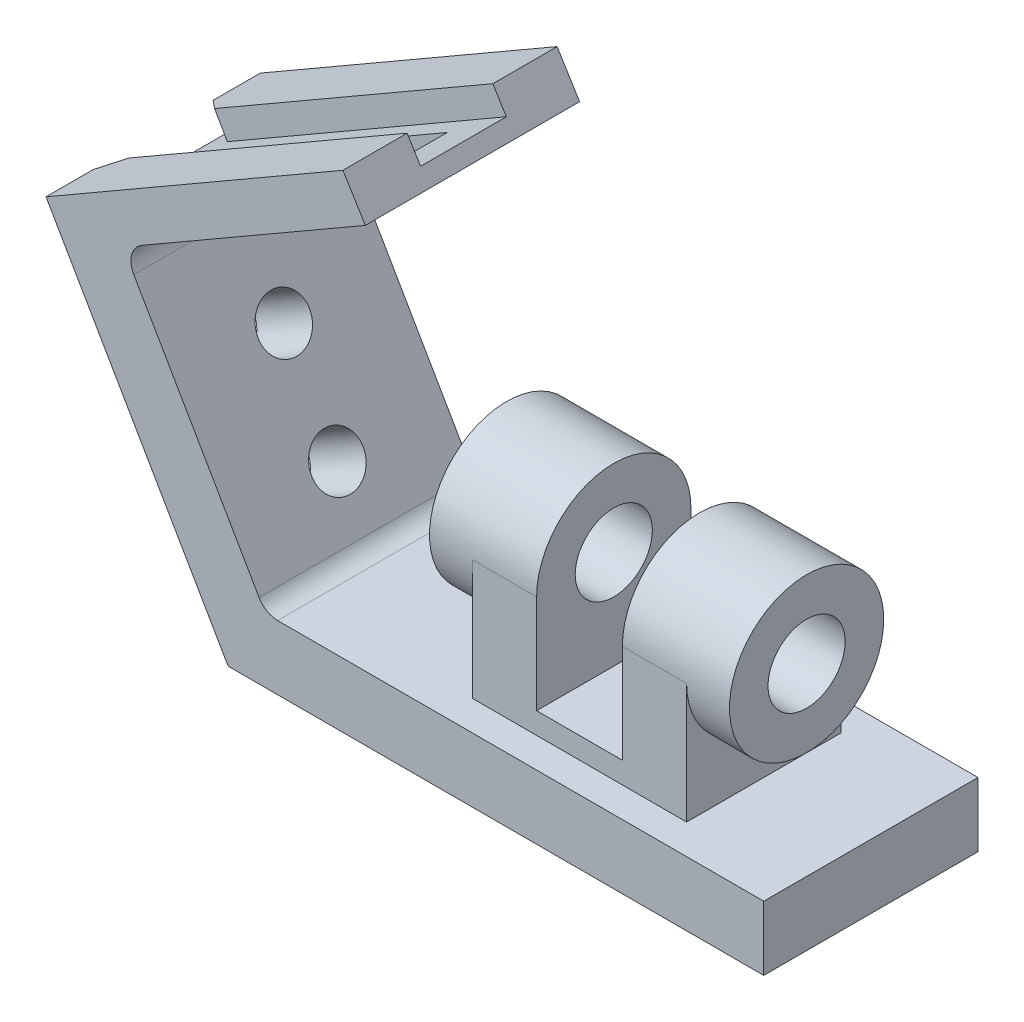
ISO-10303-21;
HEADER;
FILE_DESCRIPTION(('STEP AP214'),'2;1');
FILE_NAME('part.step','',(''),(''),'','','');
FILE_SCHEMA(('AUTOMOTIVE_DESIGN { 1 0 10303 214 1 1 1 1 }'));
ENDSEC;
DATA;
#1=APPLICATION_CONTEXT('core data for automotive mechanical design processes');
#2=APPLICATION_PROTOCOL_DEFINITION('international standard','automotive_design',2000,#1);
#3=PRODUCT_CONTEXT('',#1,'mechanical');
#4=PRODUCT('Part','Part','',(#3));
#5=PRODUCT_RELATED_PRODUCT_CATEGORY('part','',(#4));
#6=PRODUCT_DEFINITION_FORMATION('','',#4);
#7=PRODUCT_DEFINITION_CONTEXT('part definition',#1,'design');
#8=PRODUCT_DEFINITION('design','',#6,#7);
#9=PRODUCT_DEFINITION_SHAPE('','',#8);
#10=(LENGTH_UNIT() NAMED_UNIT(*) SI_UNIT(.MILLI.,.METRE.));
#11=(NAMED_UNIT(*) PLANE_ANGLE_UNIT() SI_UNIT($,.RADIAN.));
#12=(NAMED_UNIT(*) SI_UNIT($,.STERADIAN.) SOLID_ANGLE_UNIT());
#13=UNCERTAINTY_MEASURE_WITH_UNIT(LENGTH_MEASURE(1.E-05),#10,'distance_accuracy_value','');
#14=(GEOMETRIC_REPRESENTATION_CONTEXT(3) GLOBAL_UNCERTAINTY_ASSIGNED_CONTEXT((#13)) GLOBAL_UNIT_ASSIGNED_CONTEXT((#10,
#11,#12)) REPRESENTATION_CONTEXT('',''));
#15=CARTESIAN_POINT('',(0.,0.,0.));
#16=DIRECTION('',(0.,0.,1.));
#17=DIRECTION('',(1.,0.,0.));
#18=AXIS2_PLACEMENT_3D('',#15,#16,#17);
#19=CARTESIAN_POINT('',(40.,43.,0.));
#20=DIRECTION('',(1.,0.,0.));
#21=DIRECTION('',(0.,0.,-1.));
#22=AXIS2_PLACEMENT_3D('',#19,#20,#21);
#23=CYLINDRICAL_SURFACE('',#22,18.);
#24=CARTESIAN_POINT('',(85.,43.,0.));
#25=DIRECTION('',(1.,0.,0.));
#26=DIRECTION('',(0.,1.,0.));
#27=AXIS2_PLACEMENT_3D('',#24,#25,#26);
#28=CIRCLE('',#27,18.);
#29=CARTESIAN_POINT('',(85.,43.,18.));
#30=VERTEX_POINT('',#29);
#31=CARTESIAN_POINT('',(85.,43.,-18.));
#32=VERTEX_POINT('',#31);
#33=EDGE_CURVE('E48',#30,#32,#28,.F.);
#34=ORIENTED_EDGE('',*,*,#33,.F.);
#35=DIRECTION('',(1.,0.,0.));
#36=VECTOR('',#35,1.);
#37=CARTESIAN_POINT('',(50.,43.,18.));
#38=LINE('',#37,#36);
#39=CARTESIAN_POINT('',(100.,43.,18.));
#40=VERTEX_POINT('',#39);
#41=EDGE_CURVE('E285',#30,#40,#38,.T.);
#42=ORIENTED_EDGE('',*,*,#41,.T.);
#43=CARTESIAN_POINT('',(100.,43.,0.));
#44=DIRECTION('',(-1.,0.,0.));
#45=DIRECTION('',(0.,0.,1.));
#46=AXIS2_PLACEMENT_3D('',#43,#44,#45);
#47=CIRCLE('',#46,18.);
#48=CARTESIAN_POINT('',(100.,43.,-18.));
#49=VERTEX_POINT('',#48);
#50=EDGE_CURVE('E434',#49,#40,#47,.T.);
#51=ORIENTED_EDGE('',*,*,#50,.F.);
#52=DIRECTION('',(1.,0.,0.));
#53=VECTOR('',#52,1.);
#54=CARTESIAN_POINT('',(50.,43.,-18.));
#55=LINE('',#54,#53);
#56=EDGE_CURVE('E276',#32,#49,#55,.T.);
#57=ORIENTED_EDGE('',*,*,#56,.F.);
#58=EDGE_LOOP('',(#34,#42,#51,#57));
#59=FACE_BOUND('',#58,.T.);
#60=CARTESIAN_POINT('',(110.,43.,0.));
#61=DIRECTION('',(1.,0.,0.));
#62=DIRECTION('',(0.,0.,-1.));
#63=AXIS2_PLACEMENT_3D('',#60,#61,#62);
#64=CIRCLE('',#63,18.);
#65=CARTESIAN_POINT('',(110.,43.,-18.));
#66=VERTEX_POINT('',#65);
#67=EDGE_CURVE('E255',#66,#66,#64,.T.);
#68=ORIENTED_EDGE('',*,*,#67,.F.);
#69=EDGE_LOOP('',(#68));
#70=FACE_BOUND('',#69,.T.);
#71=ADVANCED_FACE('F39',(#59,#70),#23,.T.);
#72=CARTESIAN_POINT('',(-42.5000000000004,73.6121593216771,25.));
#73=DIRECTION('',(0.500000000000004,-0.866025403784436,0.));
#74=DIRECTION('',(0.866025403784436,0.500000000000004,0.));
#75=AXIS2_PLACEMENT_3D('',#72,#73,#74);
#76=PLANE('',#75);
#77=DIRECTION('',(0.,0.,-1.));
#78=VECTOR('',#77,1.);
#79=CARTESIAN_POINT('',(-42.5000000000004,73.6121593216771,25.));
#80=LINE('',#79,#78);
#81=CARTESIAN_POINT('',(-42.5000000000004,73.6121593216771,-14.));
#82=VERTEX_POINT('',#81);
#83=CARTESIAN_POINT('',(-42.5000000000004,73.6121593216771,-25.));
#84=VERTEX_POINT('',#83);
#85=EDGE_CURVE('E410',#82,#84,#80,.T.);
#86=ORIENTED_EDGE('',*,*,#85,.F.);
#87=DIRECTION('',(-0.676252226000572,-0.39043440472152,-0.624695047554424));
#88=VECTOR('',#87,1.);
#89=CARTESIAN_POINT('',(-42.5000000000004,73.6121593216771,-14.));
#90=LINE('',#89,#88);
#91=CARTESIAN_POINT('',(-38.1698729810782,76.1121593216771,-10.));
#92=VERTEX_POINT('',#91);
#93=EDGE_CURVE('E316',#92,#82,#90,.T.);
#94=ORIENTED_EDGE('',*,*,#93,.F.);
#95=DIRECTION('',(0.866025403784436,0.500000000000004,0.));
#96=VECTOR('',#95,1.);
#97=CARTESIAN_POINT('',(-38.1698729810782,76.1121593216771,-10.));
#98=LINE('',#97,#96);
#99=CARTESIAN_POINT('',(26.7820323027545,113.612159321677,-10.));
#100=VERTEX_POINT('',#99);
#101=EDGE_CURVE('E342',#92,#100,#98,.T.);
#102=ORIENTED_EDGE('',*,*,#101,.T.);
#103=DIRECTION('',(0.,0.,-1.));
#104=VECTOR('',#103,1.);
#105=CARTESIAN_POINT('',(26.7820323027545,113.612159321677,25.));
#106=LINE('',#105,#104);
#107=CARTESIAN_POINT('',(26.7820323027545,113.612159321677,-25.));
#108=VERTEX_POINT('',#107);
#109=EDGE_CURVE('E414',#100,#108,#106,.T.);
#110=ORIENTED_EDGE('',*,*,#109,.T.);
#111=DIRECTION('',(-0.866025403784436,-0.500000000000004,0.));
#112=VECTOR('',#111,1.);
#113=CARTESIAN_POINT('',(-42.5000000000004,73.6121593216771,-25.));
#114=LINE('',#113,#112);
#115=EDGE_CURVE('E396',#108,#84,#114,.T.);
#116=ORIENTED_EDGE('',*,*,#115,.T.);
#117=EDGE_LOOP('',(#86,#94,#102,#110,#116));
#118=FACE_BOUND('',#117,.T.);
#119=ADVANCED_FACE('F478',(#118),#76,.F.);
#120=CARTESIAN_POINT('',(32.0205297038397,105.094052432302,25.));
#121=DIRECTION('',(-0.851810688937537,-0.523849740108516,0.));
#122=DIRECTION('',(0.523849740108516,-0.851810688937537,0.));
#123=AXIS2_PLACEMENT_3D('',#120,#121,#122);
#124=PLANE('',#123);
#125=DIRECTION('',(-0.523849740108516,0.851810688937537,0.));
#126=VECTOR('',#125,1.);
#127=CARTESIAN_POINT('',(32.0205297038397,105.094052432302,-9.99999999999999));
#128=LINE('',#127,#126);
#129=CARTESIAN_POINT('',(29.926342667875,108.49932452712,-10.));
#130=VERTEX_POINT('',#129);
#131=EDGE_CURVE('E355',#130,#100,#128,.T.);
#132=ORIENTED_EDGE('',*,*,#131,.F.);
#133=DIRECTION('',(0.,0.,-1.));
#134=VECTOR('',#133,1.);
#135=CARTESIAN_POINT('',(29.926342667875,108.49932452712,25.));
#136=LINE('',#135,#134);
#137=CARTESIAN_POINT('',(29.926342667875,108.49932452712,10.));
#138=VERTEX_POINT('',#137);
#139=EDGE_CURVE('E433',#138,#130,#136,.T.);
#140=ORIENTED_EDGE('',*,*,#139,.F.);
#141=DIRECTION('',(-0.523849740108516,0.851810688937537,0.));
#142=VECTOR('',#141,1.);
#143=CARTESIAN_POINT('',(32.0205297038397,105.094052432302,10.));
#144=LINE('',#143,#142);
#145=CARTESIAN_POINT('',(26.7820323027545,113.612159321677,10.));
#146=VERTEX_POINT('',#145);
#147=EDGE_CURVE('E347',#138,#146,#144,.T.);
#148=ORIENTED_EDGE('',*,*,#147,.T.);
#149=CARTESIAN_POINT('',(26.7820323027545,113.612159321677,25.));
#150=VERTEX_POINT('',#149);
#151=EDGE_CURVE('E411',#150,#146,#106,.T.);
#152=ORIENTED_EDGE('',*,*,#151,.F.);
#153=DIRECTION('',(-0.523849740108516,0.851810688937537,0.));
#154=VECTOR('',#153,1.);
#155=CARTESIAN_POINT('',(32.0205297038397,105.094052432302,25.));
#156=LINE('',#155,#154);
#157=CARTESIAN_POINT('',(32.0205297038397,105.094052432302,25.));
#158=VERTEX_POINT('',#157);
#159=EDGE_CURVE('E375',#158,#150,#156,.T.);
#160=ORIENTED_EDGE('',*,*,#159,.F.);
#161=DIRECTION('',(0.,0.,-1.));
#162=VECTOR('',#161,1.);
#163=CARTESIAN_POINT('',(32.0205297038397,105.094052432302,25.));
#164=LINE('',#163,#162);
#165=CARTESIAN_POINT('',(32.0205297038397,105.094052432302,-25.));
#166=VERTEX_POINT('',#165);
#167=EDGE_CURVE('E412',#158,#166,#164,.T.);
#168=ORIENTED_EDGE('',*,*,#167,.T.);
#169=DIRECTION('',(-0.523849740108516,0.851810688937537,0.));
#170=VECTOR('',#169,1.);
#171=CARTESIAN_POINT('',(32.0205297038397,105.094052432302,-25.));
#172=LINE('',#171,#170);
#173=EDGE_CURVE('E395',#166,#108,#172,.T.);
#174=ORIENTED_EDGE('',*,*,#173,.T.);
#175=ORIENTED_EDGE('',*,*,#109,.F.);
#176=EDGE_LOOP('',(#132,#140,#148,#152,#160,#168,#174,#175));
#177=FACE_BOUND('',#176,.T.);
#178=ADVANCED_FACE('F485',(#177),#124,.F.);
#179=DIRECTION('',(0.866025403784436,0.500000000000004,0.));
#180=VECTOR('',#179,1.);
#181=CARTESIAN_POINT('',(-38.1698729810782,76.1121593216771,10.));
#182=LINE('',#181,#180);
#183=CARTESIAN_POINT('',(-38.1698729810782,76.1121593216771,10.));
#184=VERTEX_POINT('',#183);
#185=EDGE_CURVE('E333',#184,#146,#182,.T.);
#186=ORIENTED_EDGE('',*,*,#185,.F.);
#187=DIRECTION('',(0.676252226000572,0.390434404721518,-0.624695047554425));
#188=VECTOR('',#187,1.);
#189=CARTESIAN_POINT('',(-38.1698729810782,76.1121593216771,10.));
#190=LINE('',#189,#188);
#191=CARTESIAN_POINT('',(-42.5000000000004,73.6121593216771,14.));
#192=VERTEX_POINT('',#191);
#193=EDGE_CURVE('E321',#192,#184,#190,.T.);
#194=ORIENTED_EDGE('',*,*,#193,.F.);
#195=CARTESIAN_POINT('',(-42.5000000000004,73.6121593216771,25.));
#196=VERTEX_POINT('',#195);
#197=EDGE_CURVE('E409',#196,#192,#80,.T.);
#198=ORIENTED_EDGE('',*,*,#197,.F.);
#199=DIRECTION('',(-0.866025403784436,-0.500000000000004,0.));
#200=VECTOR('',#199,1.);
#201=CARTESIAN_POINT('',(-42.5000000000004,73.6121593216771,25.));
#202=LINE('',#201,#200);
#203=EDGE_CURVE('E372',#150,#196,#202,.T.);
#204=ORIENTED_EDGE('',*,*,#203,.F.);
#205=ORIENTED_EDGE('',*,*,#151,.T.);
#206=EDGE_LOOP('',(#186,#194,#198,#204,#205));
#207=FACE_BOUND('',#206,.T.);
#208=ADVANCED_FACE('F486',(#207),#76,.F.);
#209=CARTESIAN_POINT('',(125.,0.,25.));
#210=DIRECTION('',(-1.,0.,0.));
#211=DIRECTION('',(0.,0.,1.));
#212=AXIS2_PLACEMENT_3D('',#209,#210,#211);
#213=PLANE('',#212);
#214=DIRECTION('',(0.,1.,0.));
#215=VECTOR('',#214,1.);
#216=CARTESIAN_POINT('',(125.,0.,-25.));
#217=LINE('',#216,#215);
#218=CARTESIAN_POINT('',(125.,0.,-25.));
#219=VERTEX_POINT('',#218);
#220=CARTESIAN_POINT('',(125.,15.,-25.));
#221=VERTEX_POINT('',#220);
#222=EDGE_CURVE('E357',#219,#221,#217,.T.);
#223=ORIENTED_EDGE('',*,*,#222,.T.);
#224=DIRECTION('',(0.,0.,-1.));
#225=VECTOR('',#224,1.);
#226=CARTESIAN_POINT('',(125.,15.,25.));
#227=LINE('',#226,#225);
#228=CARTESIAN_POINT('',(125.,15.,25.));
#229=VERTEX_POINT('',#228);
#230=EDGE_CURVE('E427',#229,#221,#227,.T.);
#231=ORIENTED_EDGE('',*,*,#230,.F.);
#232=DIRECTION('',(0.,1.,0.));
#233=VECTOR('',#232,1.);
#234=CARTESIAN_POINT('',(125.,0.,25.));
#235=LINE('',#234,#233);
#236=CARTESIAN_POINT('',(125.,0.,25.));
#237=VERTEX_POINT('',#236);
#238=EDGE_CURVE('E356',#237,#229,#235,.T.);
#239=ORIENTED_EDGE('',*,*,#238,.F.);
#240=DIRECTION('',(0.,0.,-1.));
#241=VECTOR('',#240,1.);
#242=CARTESIAN_POINT('',(125.,0.,25.));
#243=LINE('',#242,#241);
#244=EDGE_CURVE('E379',#237,#219,#243,.T.);
#245=ORIENTED_EDGE('',*,*,#244,.T.);
#246=EDGE_LOOP('',(#223,#231,#239,#245));
#247=FACE_BOUND('',#246,.T.);
#248=ADVANCED_FACE('F41',(#247),#213,.F.);
#249=CARTESIAN_POINT('',(125.,15.,25.));
#250=DIRECTION('',(0.,-1.,0.));
#251=DIRECTION('',(1.,0.,0.));
#252=AXIS2_PLACEMENT_3D('',#249,#250,#251);
#253=PLANE('',#252);
#254=DIRECTION('',(1.,0.,0.));
#255=VECTOR('',#254,1.);
#256=CARTESIAN_POINT('',(50.,15.,18.));
#257=LINE('',#256,#255);
#258=CARTESIAN_POINT('',(50.,15.,18.));
#259=VERTEX_POINT('',#258);
#260=CARTESIAN_POINT('',(100.,15.,18.));
#261=VERTEX_POINT('',#260);
#262=EDGE_CURVE('E64',#259,#261,#257,.T.);
#263=ORIENTED_EDGE('',*,*,#262,.F.);
#264=DIRECTION('',(0.,0.,1.));
#265=VECTOR('',#264,1.);
#266=CARTESIAN_POINT('',(50.,15.,-18.));
#267=LINE('',#266,#265);
#268=CARTESIAN_POINT('',(50.,15.,-18.));
#269=VERTEX_POINT('',#268);
#270=EDGE_CURVE('E264',#269,#259,#267,.T.);
#271=ORIENTED_EDGE('',*,*,#270,.F.);
#272=DIRECTION('',(1.,0.,0.));
#273=VECTOR('',#272,1.);
#274=CARTESIAN_POINT('',(50.,15.,-18.));
#275=LINE('',#274,#273);
#276=CARTESIAN_POINT('',(100.,15.,-18.));
#277=VERTEX_POINT('',#276);
#278=EDGE_CURVE('E272',#269,#277,#275,.T.);
#279=ORIENTED_EDGE('',*,*,#278,.T.);
#280=DIRECTION('',(0.,0.,1.));
#281=VECTOR('',#280,1.);
#282=CARTESIAN_POINT('',(100.,15.,-18.));
#283=LINE('',#282,#281);
#284=EDGE_CURVE('E258',#277,#261,#283,.T.);
#285=ORIENTED_EDGE('',*,*,#284,.T.);
#286=EDGE_LOOP('',(#263,#271,#279,#285));
#287=FACE_BOUND('',#286,.T.);
#288=DIRECTION('',(-1.,0.,0.));
#289=VECTOR('',#288,1.);
#290=CARTESIAN_POINT('',(125.,15.,-25.));
#291=LINE('',#290,#289);
#292=CARTESIAN_POINT('',(11.5470053837925,15.,-25.));
#293=VERTEX_POINT('',#292);
#294=EDGE_CURVE('E384',#221,#293,#291,.T.);
#295=ORIENTED_EDGE('',*,*,#294,.T.);
#296=DIRECTION('',(0.,0.,-1.));
#297=VECTOR('',#296,1.);
#298=CARTESIAN_POINT('',(11.5470053837925,15.,25.));
#299=LINE('',#298,#297);
#300=CARTESIAN_POINT('',(11.5470053837925,15.,25.));
#301=VERTEX_POINT('',#300);
#302=EDGE_CURVE('E430',#301,#293,#299,.T.);
#303=ORIENTED_EDGE('',*,*,#302,.F.);
#304=DIRECTION('',(-1.,0.,0.));
#305=VECTOR('',#304,1.);
#306=CARTESIAN_POINT('',(125.,15.,25.));
#307=LINE('',#306,#305);
#308=EDGE_CURVE('E363',#229,#301,#307,.T.);
#309=ORIENTED_EDGE('',*,*,#308,.F.);
#310=ORIENTED_EDGE('',*,*,#230,.T.);
#311=EDGE_LOOP('',(#295,#303,#309,#310));
#312=FACE_BOUND('',#311,.T.);
#313=ADVANCED_FACE('F570',(#287,#312),#253,.F.);
#314=CARTESIAN_POINT('',(11.5470053837924,20.,25.));
#315=DIRECTION('',(0.,0.,-1.));
#316=DIRECTION('',(-1.,0.,0.));
#317=AXIS2_PLACEMENT_3D('',#314,#315,#316);
#318=CYLINDRICAL_SURFACE('',#317,5.);
#319=CARTESIAN_POINT('',(11.5470053837924,20.,-25.));
#320=DIRECTION('',(0.,0.,-1.));
#321=DIRECTION('',(-1.,0.,0.));
#322=AXIS2_PLACEMENT_3D('',#319,#320,#321);
#323=CIRCLE('',#322,5.);
#324=CARTESIAN_POINT('',(7.21687836487027,17.5,-25.));
#325=VERTEX_POINT('',#324);
#326=EDGE_CURVE('E383',#293,#325,#323,.T.);
#327=ORIENTED_EDGE('',*,*,#326,.T.);
#328=DIRECTION('',(0.,0.,-1.));
#329=VECTOR('',#328,1.);
#330=CARTESIAN_POINT('',(7.21687836487027,17.5,25.));
#331=LINE('',#330,#329);
#332=CARTESIAN_POINT('',(7.21687836487027,17.5,25.));
#333=VERTEX_POINT('',#332);
#334=EDGE_CURVE('E425',#333,#325,#331,.T.);
#335=ORIENTED_EDGE('',*,*,#334,.F.);
#336=CARTESIAN_POINT('',(11.5470053837924,20.,25.));
#337=DIRECTION('',(0.,0.,-1.));
#338=DIRECTION('',(-1.,0.,0.));
#339=AXIS2_PLACEMENT_3D('',#336,#337,#338);
#340=CIRCLE('',#339,5.);
#341=EDGE_CURVE('E364',#301,#333,#340,.T.);
#342=ORIENTED_EDGE('',*,*,#341,.F.);
#343=ORIENTED_EDGE('',*,*,#302,.T.);
#344=EDGE_LOOP('',(#327,#335,#342,#343));
#345=FACE_BOUND('',#344,.T.);
#346=ADVANCED_FACE('F562',(#345),#318,.F.);
#347=CARTESIAN_POINT('',(7.21687836487027,17.5,25.));
#348=DIRECTION('',(-0.866025403784436,-0.500000000000004,0.));
#349=DIRECTION('',(0.500000000000004,-0.866025403784436,0.));
#350=AXIS2_PLACEMENT_3D('',#347,#348,#349);
#351=PLANE('',#350);
#352=CARTESIAN_POINT('',(0.49038105676642,29.150635094611,0.));
#353=DIRECTION('',(-0.866025403784436,-0.500000000000004,0.));
#354=DIRECTION('',(0.500000000000004,-0.866025403784436,0.));
#355=AXIS2_PLACEMENT_3D('',#352,#353,#354);
#356=CIRCLE('',#355,6.);
#357=CARTESIAN_POINT('',(3.49038105676645,23.9544826719044,0.));
#358=VERTEX_POINT('',#357);
#359=EDGE_CURVE('E835',#358,#358,#356,.T.);
#360=ORIENTED_EDGE('',*,*,#359,.T.);
#361=EDGE_LOOP('',(#360));
#362=FACE_BOUND('',#361,.T.);
#363=CARTESIAN_POINT('',(-12.0096189432337,50.8012701892219,0.));
#364=DIRECTION('',(-0.866025403784436,-0.500000000000004,0.));
#365=DIRECTION('',(0.500000000000004,-0.866025403784436,0.));
#366=AXIS2_PLACEMENT_3D('',#363,#364,#365);
#367=CIRCLE('',#366,6.);
#368=CARTESIAN_POINT('',(-9.00961894323366,45.6051177665153,0.));
#369=VERTEX_POINT('',#368);
#370=EDGE_CURVE('E833',#369,#369,#367,.T.);
#371=ORIENTED_EDGE('',*,*,#370,.T.);
#372=EDGE_LOOP('',(#371));
#373=FACE_BOUND('',#372,.T.);
#374=DIRECTION('',(-0.500000000000004,0.866025403784436,0.));
#375=VECTOR('',#374,1.);
#376=CARTESIAN_POINT('',(7.21687836487027,17.5,-25.));
#377=LINE('',#376,#375);
#378=CARTESIAN_POINT('',(-22.0115461137875,68.1251162222244,-25.));
#379=VERTEX_POINT('',#378);
#380=EDGE_CURVE('E390',#325,#379,#377,.T.);
#381=ORIENTED_EDGE('',*,*,#380,.T.);
#382=DIRECTION('',(0.,0.,-1.));
#383=VECTOR('',#382,1.);
#384=CARTESIAN_POINT('',(-22.0115461137875,68.1251162222244,25.));
#385=LINE('',#384,#383);
#386=CARTESIAN_POINT('',(-22.0115461137875,68.1251162222244,25.));
#387=VERTEX_POINT('',#386);
#388=EDGE_CURVE('E423',#387,#379,#385,.T.);
#389=ORIENTED_EDGE('',*,*,#388,.F.);
#390=DIRECTION('',(-0.500000000000004,0.866025403784436,0.));
#391=VECTOR('',#390,1.);
#392=CARTESIAN_POINT('',(7.21687836487027,17.5,25.));
#393=LINE('',#392,#391);
#394=EDGE_CURVE('E366',#333,#387,#393,.T.);
#395=ORIENTED_EDGE('',*,*,#394,.F.);
#396=ORIENTED_EDGE('',*,*,#334,.T.);
#397=EDGE_LOOP('',(#381,#389,#395,#396));
#398=FACE_BOUND('',#397,.T.);
#399=ADVANCED_FACE('F557',(#362,#373,#398),#351,.F.);
#400=CARTESIAN_POINT('',(-17.6814190948651,70.6251162222242,25.));
#401=DIRECTION('',(0.,0.,-1.));
#402=DIRECTION('',(-1.,0.,0.));
#403=AXIS2_PLACEMENT_3D('',#400,#401,#402);
#404=CYLINDRICAL_SURFACE('',#403,5.0000000000001);
#405=CARTESIAN_POINT('',(-17.6814190948651,70.6251162222242,-25.));
#406=DIRECTION('',(0.,0.,-1.));
#407=DIRECTION('',(-1.,0.,0.));
#408=AXIS2_PLACEMENT_3D('',#405,#406,#407);
#409=CIRCLE('',#408,5.0000000000001);
#410=CARTESIAN_POINT('',(-20.1814190948653,74.9552432411466,-25.));
#411=VERTEX_POINT('',#410);
#412=EDGE_CURVE('E386',#379,#411,#409,.T.);
#413=ORIENTED_EDGE('',*,*,#412,.T.);
#414=DIRECTION('',(0.,0.,-1.));
#415=VECTOR('',#414,1.);
#416=CARTESIAN_POINT('',(-20.1814190948653,74.9552432411466,25.));
#417=LINE('',#416,#415);
#418=CARTESIAN_POINT('',(-20.1814190948653,74.9552432411466,25.));
#419=VERTEX_POINT('',#418);
#420=EDGE_CURVE('E419',#419,#411,#417,.T.);
#421=ORIENTED_EDGE('',*,*,#420,.F.);
#422=CARTESIAN_POINT('',(-17.6814190948651,70.6251162222242,25.));
#423=DIRECTION('',(0.,0.,-1.));
#424=DIRECTION('',(-1.,0.,0.));
#425=AXIS2_PLACEMENT_3D('',#422,#423,#424);
#426=CIRCLE('',#425,5.0000000000001);
#427=EDGE_CURVE('E368',#387,#419,#426,.T.);
#428=ORIENTED_EDGE('',*,*,#427,.F.);
#429=ORIENTED_EDGE('',*,*,#388,.T.);
#430=EDGE_LOOP('',(#413,#421,#428,#429));
#431=FACE_BOUND('',#430,.T.);
#432=ADVANCED_FACE('F558',(#431),#404,.F.);
#433=CARTESIAN_POINT('',(-20.1814190948653,74.9552432411466,25.));
#434=DIRECTION('',(-0.500000000000001,0.866025403784438,0.));
#435=DIRECTION('',(-0.866025403784438,-0.500000000000001,0.));
#436=AXIS2_PLACEMENT_3D('',#433,#434,#435);
#437=PLANE('',#436);
#438=DIRECTION('',(0.866025403784438,0.500000000000001,0.));
#439=VECTOR('',#438,1.);
#440=CARTESIAN_POINT('',(-20.1814190948653,74.9552432411466,5.));
#441=LINE('',#440,#439);
#442=CARTESIAN_POINT('',(-11.5211650570209,79.9552432411466,5.));
#443=VERTEX_POINT('',#442);
#444=CARTESIAN_POINT('',(23.1198510943566,99.9552432411466,5.00000000000001));
#445=VERTEX_POINT('',#444);
#446=EDGE_CURVE('E312',#443,#445,#441,.T.);
#447=ORIENTED_EDGE('',*,*,#446,.T.);
#448=DIRECTION('',(0.,0.,-1.));
#449=VECTOR('',#448,1.);
#450=CARTESIAN_POINT('',(23.1198510943566,99.9552432411466,25.));
#451=LINE('',#450,#449);
#452=CARTESIAN_POINT('',(23.1198510943566,99.9552432411466,-4.99999999999999));
#453=VERTEX_POINT('',#452);
#454=EDGE_CURVE('E317',#445,#453,#451,.T.);
#455=ORIENTED_EDGE('',*,*,#454,.T.);
#456=DIRECTION('',(-0.866025403784438,-0.500000000000001,0.));
#457=VECTOR('',#456,1.);
#458=CARTESIAN_POINT('',(-20.1814190948653,74.9552432411466,-5.));
#459=LINE('',#458,#457);
#460=CARTESIAN_POINT('',(-11.5211650570209,79.9552432411466,-5.));
#461=VERTEX_POINT('',#460);
#462=EDGE_CURVE('E301',#453,#461,#459,.T.);
#463=ORIENTED_EDGE('',*,*,#462,.T.);
#464=DIRECTION('',(0.,0.,1.));
#465=VECTOR('',#464,1.);
#466=CARTESIAN_POINT('',(-11.5211650570209,79.9552432411466,25.));
#467=LINE('',#466,#465);
#468=EDGE_CURVE('E309',#461,#443,#467,.T.);
#469=ORIENTED_EDGE('',*,*,#468,.T.);
#470=EDGE_LOOP('',(#447,#455,#463,#469));
#471=FACE_BOUND('',#470,.T.);
#472=DIRECTION('',(0.866025403784438,0.500000000000001,0.));
#473=VECTOR('',#472,1.);
#474=CARTESIAN_POINT('',(-20.1814190948653,74.9552432411466,-25.));
#475=LINE('',#474,#473);
#476=EDGE_CURVE('E394',#411,#166,#475,.T.);
#477=ORIENTED_EDGE('',*,*,#476,.T.);
#478=ORIENTED_EDGE('',*,*,#167,.F.);
#479=DIRECTION('',(0.866025403784438,0.500000000000001,0.));
#480=VECTOR('',#479,1.);
#481=CARTESIAN_POINT('',(-20.1814190948653,74.9552432411466,25.));
#482=LINE('',#481,#480);
#483=EDGE_CURVE('E369',#419,#158,#482,.T.);
#484=ORIENTED_EDGE('',*,*,#483,.F.);
#485=ORIENTED_EDGE('',*,*,#420,.T.);
#486=EDGE_LOOP('',(#477,#478,#484,#485));
#487=FACE_BOUND('',#486,.T.);
#488=ADVANCED_FACE('F546',(#471,#487),#437,.F.);
#489=CARTESIAN_POINT('',(0.,0.,25.));
#490=DIRECTION('',(0.866025403784436,0.500000000000004,0.));
#491=DIRECTION('',(-0.500000000000004,0.866025403784436,0.));
#492=AXIS2_PLACEMENT_3D('',#489,#490,#491);
#493=PLANE('',#492);
#494=CARTESIAN_POINT('',(-12.5000000000001,21.6506350946109,0.));
#495=DIRECTION('',(-0.866025403784436,-0.500000000000004,0.));
#496=DIRECTION('',(0.500000000000004,-0.866025403784436,0.));
#497=AXIS2_PLACEMENT_3D('',#494,#495,#496);
#498=CIRCLE('',#497,6.);
#499=CARTESIAN_POINT('',(-9.50000000000009,16.4544826719043,0.));
#500=VERTEX_POINT('',#499);
#501=EDGE_CURVE('E827',#500,#500,#498,.T.);
#502=ORIENTED_EDGE('',*,*,#501,.F.);
#503=EDGE_LOOP('',(#502));
#504=FACE_BOUND('',#503,.T.);
#505=CARTESIAN_POINT('',(-25.0000000000002,43.3012701892218,0.));
#506=DIRECTION('',(-0.866025403784436,-0.500000000000004,0.));
#507=DIRECTION('',(0.500000000000004,-0.866025403784436,0.));
#508=AXIS2_PLACEMENT_3D('',#505,#506,#507);
#509=CIRCLE('',#508,6.);
#510=CARTESIAN_POINT('',(-22.0000000000002,38.1051177665152,0.));
#511=VERTEX_POINT('',#510);
#512=EDGE_CURVE('E836',#511,#511,#509,.T.);
#513=ORIENTED_EDGE('',*,*,#512,.F.);
#514=EDGE_LOOP('',(#513));
#515=FACE_BOUND('',#514,.T.);
#516=DIRECTION('',(0.,0.,1.));
#517=VECTOR('',#516,1.);
#518=CARTESIAN_POINT('',(-39.5000000000003,68.4160068989705,-14.));
#519=LINE('',#518,#517);
#520=CARTESIAN_POINT('',(-39.5000000000003,68.4160068989705,-14.));
#521=VERTEX_POINT('',#520);
#522=CARTESIAN_POINT('',(-39.5000000000003,68.4160068989705,14.));
#523=VERTEX_POINT('',#522);
#524=EDGE_CURVE('E324',#521,#523,#519,.T.);
#525=ORIENTED_EDGE('',*,*,#524,.F.);
#526=DIRECTION('',(-0.500000000000004,0.866025403784436,0.));
#527=VECTOR('',#526,1.);
#528=CARTESIAN_POINT('',(-39.5000000000003,68.4160068989705,-14.));
#529=LINE('',#528,#527);
#530=EDGE_CURVE('E328',#521,#82,#529,.T.);
#531=ORIENTED_EDGE('',*,*,#530,.T.);
#532=ORIENTED_EDGE('',*,*,#85,.T.);
#533=DIRECTION('',(0.500000000000004,-0.866025403784436,0.));
#534=VECTOR('',#533,1.);
#535=CARTESIAN_POINT('',(0.,0.,-25.));
#536=LINE('',#535,#534);
#537=CARTESIAN_POINT('',(0.,0.,-25.));
#538=VERTEX_POINT('',#537);
#539=EDGE_CURVE('E398',#84,#538,#536,.T.);
#540=ORIENTED_EDGE('',*,*,#539,.T.);
#541=DIRECTION('',(0.,0.,-1.));
#542=VECTOR('',#541,1.);
#543=CARTESIAN_POINT('',(0.,0.,25.));
#544=LINE('',#543,#542);
#545=CARTESIAN_POINT('',(0.,0.,25.));
#546=VERTEX_POINT('',#545);
#547=EDGE_CURVE('E404',#546,#538,#544,.T.);
#548=ORIENTED_EDGE('',*,*,#547,.F.);
#549=DIRECTION('',(0.500000000000004,-0.866025403784436,0.));
#550=VECTOR('',#549,1.);
#551=CARTESIAN_POINT('',(0.,0.,25.));
#552=LINE('',#551,#550);
#553=EDGE_CURVE('E376',#196,#546,#552,.T.);
#554=ORIENTED_EDGE('',*,*,#553,.F.);
#555=ORIENTED_EDGE('',*,*,#197,.T.);
#556=DIRECTION('',(-0.500000000000004,0.866025403784436,0.));
#557=VECTOR('',#556,1.);
#558=CARTESIAN_POINT('',(-39.5000000000003,68.4160068989705,14.));
#559=LINE('',#558,#557);
#560=EDGE_CURVE('E332',#523,#192,#559,.T.);
#561=ORIENTED_EDGE('',*,*,#560,.F.);
#562=EDGE_LOOP('',(#525,#531,#532,#540,#548,#554,#555,#561));
#563=FACE_BOUND('',#562,.T.);
#564=ADVANCED_FACE('F545',(#504,#515,#563),#493,.F.);
#565=CARTESIAN_POINT('',(125.,0.,25.));
#566=DIRECTION('',(0.,1.,0.));
#567=DIRECTION('',(0.,0.,1.));
#568=AXIS2_PLACEMENT_3D('',#565,#566,#567);
#569=PLANE('',#568);
#570=DIRECTION('',(1.,0.,0.));
#571=VECTOR('',#570,1.);
#572=CARTESIAN_POINT('',(125.,0.,-25.));
#573=LINE('',#572,#571);
#574=EDGE_CURVE('E365',#538,#219,#573,.T.);
#575=ORIENTED_EDGE('',*,*,#574,.T.);
#576=ORIENTED_EDGE('',*,*,#244,.F.);
#577=DIRECTION('',(1.,0.,0.));
#578=VECTOR('',#577,1.);
#579=CARTESIAN_POINT('',(125.,0.,25.));
#580=LINE('',#579,#578);
#581=EDGE_CURVE('E377',#546,#237,#580,.T.);
#582=ORIENTED_EDGE('',*,*,#581,.F.);
#583=ORIENTED_EDGE('',*,*,#547,.T.);
#584=EDGE_LOOP('',(#575,#576,#582,#583));
#585=FACE_BOUND('',#584,.T.);
#586=ADVANCED_FACE('F537',(#585),#569,.F.);
#587=CARTESIAN_POINT('',(11.5470053837924,20.,25.));
#588=DIRECTION('',(0.,0.,-1.));
#589=DIRECTION('',(-1.,0.,0.));
#590=AXIS2_PLACEMENT_3D('',#587,#588,#589);
#591=PLANE('',#590);
#592=ORIENTED_EDGE('',*,*,#238,.T.);
#593=ORIENTED_EDGE('',*,*,#308,.T.);
#594=ORIENTED_EDGE('',*,*,#341,.T.);
#595=ORIENTED_EDGE('',*,*,#394,.T.);
#596=ORIENTED_EDGE('',*,*,#427,.T.);
#597=ORIENTED_EDGE('',*,*,#483,.T.);
#598=ORIENTED_EDGE('',*,*,#159,.T.);
#599=ORIENTED_EDGE('',*,*,#203,.T.);
#600=ORIENTED_EDGE('',*,*,#553,.T.);
#601=ORIENTED_EDGE('',*,*,#581,.T.);
#602=EDGE_LOOP('',(#592,#593,#594,#595,#596,#597,#598,#599,#600,#601));
#603=FACE_BOUND('',#602,.T.);
#604=ADVANCED_FACE('F531',(#603),#591,.F.);
#605=CARTESIAN_POINT('',(11.5470053837924,20.,-25.));
#606=DIRECTION('',(0.,0.,-1.));
#607=DIRECTION('',(-1.,0.,0.));
#608=AXIS2_PLACEMENT_3D('',#605,#606,#607);
#609=PLANE('',#608);
#610=ORIENTED_EDGE('',*,*,#222,.F.);
#611=ORIENTED_EDGE('',*,*,#574,.F.);
#612=ORIENTED_EDGE('',*,*,#539,.F.);
#613=ORIENTED_EDGE('',*,*,#115,.F.);
#614=ORIENTED_EDGE('',*,*,#173,.F.);
#615=ORIENTED_EDGE('',*,*,#476,.F.);
#616=ORIENTED_EDGE('',*,*,#412,.F.);
#617=ORIENTED_EDGE('',*,*,#380,.F.);
#618=ORIENTED_EDGE('',*,*,#326,.F.);
#619=ORIENTED_EDGE('',*,*,#294,.F.);
#620=EDGE_LOOP('',(#610,#611,#612,#613,#614,#615,#616,#617,#618,#619));
#621=FACE_BOUND('',#620,.T.);
#622=ADVANCED_FACE('F522',(#621),#609,.T.);
#623=CARTESIAN_POINT('',(-39.5000000000003,68.4160068989705,0.));
#624=DIRECTION('',(-0.500000000000004,0.866025403784436,0.));
#625=DIRECTION('',(-0.866025403784436,-0.500000000000004,0.));
#626=AXIS2_PLACEMENT_3D('',#623,#624,#625);
#627=PLANE('',#626);
#628=DIRECTION('',(0.,0.,-1.));
#629=VECTOR('',#628,1.);
#630=CARTESIAN_POINT('',(21.1217782649102,103.416006898971,-4.99999999999999));
#631=LINE('',#630,#629);
#632=CARTESIAN_POINT('',(21.1217782649102,103.416006898971,5.00000000000001));
#633=VERTEX_POINT('',#632);
#634=CARTESIAN_POINT('',(21.1217782649102,103.416006898971,-4.99999999999999));
#635=VERTEX_POINT('',#634);
#636=EDGE_CURVE('E287',#633,#635,#631,.T.);
#637=ORIENTED_EDGE('',*,*,#636,.F.);
#638=DIRECTION('',(0.866025403784436,0.500000000000004,0.));
#639=VECTOR('',#638,1.);
#640=CARTESIAN_POINT('',(-13.5192378864673,83.4160068989706,5.));
#641=LINE('',#640,#639);
#642=CARTESIAN_POINT('',(-13.5192378864673,83.4160068989706,5.));
#643=VERTEX_POINT('',#642);
#644=EDGE_CURVE('E294',#643,#633,#641,.T.);
#645=ORIENTED_EDGE('',*,*,#644,.F.);
#646=DIRECTION('',(0.,0.,1.));
#647=VECTOR('',#646,1.);
#648=CARTESIAN_POINT('',(-13.5192378864673,83.4160068989706,-5.));
#649=LINE('',#648,#647);
#650=CARTESIAN_POINT('',(-13.5192378864673,83.4160068989706,-5.));
#651=VERTEX_POINT('',#650);
#652=EDGE_CURVE('E292',#651,#643,#649,.T.);
#653=ORIENTED_EDGE('',*,*,#652,.F.);
#654=DIRECTION('',(-0.866025403784436,-0.500000000000004,0.));
#655=VECTOR('',#654,1.);
#656=CARTESIAN_POINT('',(-13.5192378864673,83.4160068989706,-5.));
#657=LINE('',#656,#655);
#658=EDGE_CURVE('E288',#635,#651,#657,.T.);
#659=ORIENTED_EDGE('',*,*,#658,.F.);
#660=EDGE_LOOP('',(#637,#645,#653,#659));
#661=FACE_BOUND('',#660,.T.);
#662=ORIENTED_EDGE('',*,*,#139,.T.);
#663=DIRECTION('',(0.866025403784436,0.500000000000004,0.));
#664=VECTOR('',#663,1.);
#665=CARTESIAN_POINT('',(-35.1698729810782,70.9160068989705,-10.));
#666=LINE('',#665,#664);
#667=CARTESIAN_POINT('',(-35.1698729810782,70.9160068989705,-10.));
#668=VERTEX_POINT('',#667);
#669=EDGE_CURVE('E338',#668,#130,#666,.T.);
#670=ORIENTED_EDGE('',*,*,#669,.F.);
#671=DIRECTION('',(-0.676252226000572,-0.39043440472152,-0.624695047554424));
#672=VECTOR('',#671,1.);
#673=CARTESIAN_POINT('',(-39.5000000000003,68.4160068989705,-14.));
#674=LINE('',#673,#672);
#675=EDGE_CURVE('E318',#668,#521,#674,.T.);
#676=ORIENTED_EDGE('',*,*,#675,.T.);
#677=ORIENTED_EDGE('',*,*,#524,.T.);
#678=DIRECTION('',(0.676252226000572,0.390434404721518,-0.624695047554425));
#679=VECTOR('',#678,1.);
#680=CARTESIAN_POINT('',(-35.1698729810782,70.9160068989705,10.));
#681=LINE('',#680,#679);
#682=CARTESIAN_POINT('',(-35.1698729810782,70.9160068989705,10.));
#683=VERTEX_POINT('',#682);
#684=EDGE_CURVE('E326',#523,#683,#681,.T.);
#685=ORIENTED_EDGE('',*,*,#684,.T.);
#686=DIRECTION('',(0.866025403784436,0.500000000000004,0.));
#687=VECTOR('',#686,1.);
#688=CARTESIAN_POINT('',(-35.1698729810782,70.9160068989705,10.));
#689=LINE('',#688,#687);
#690=EDGE_CURVE('E340',#683,#138,#689,.T.);
#691=ORIENTED_EDGE('',*,*,#690,.T.);
#692=EDGE_LOOP('',(#662,#670,#676,#677,#685,#691));
#693=FACE_BOUND('',#692,.T.);
#694=ADVANCED_FACE('F524',(#661,#693),#627,.T.);
#695=CARTESIAN_POINT('',(-35.1698729810782,70.9160068989705,-10.));
#696=DIRECTION('',(0.,0.,1.));
#697=DIRECTION('',(1.,0.,0.));
#698=AXIS2_PLACEMENT_3D('',#695,#696,#697);
#699=PLANE('',#698);
#700=ORIENTED_EDGE('',*,*,#131,.T.);
#701=ORIENTED_EDGE('',*,*,#101,.F.);
#702=DIRECTION('',(-0.500000000000004,0.866025403784436,0.));
#703=VECTOR('',#702,1.);
#704=CARTESIAN_POINT('',(-35.1698729810782,70.9160068989705,-10.));
#705=LINE('',#704,#703);
#706=EDGE_CURVE('E350',#668,#92,#705,.T.);
#707=ORIENTED_EDGE('',*,*,#706,.F.);
#708=ORIENTED_EDGE('',*,*,#669,.T.);
#709=EDGE_LOOP('',(#700,#701,#707,#708));
#710=FACE_BOUND('',#709,.T.);
#711=ADVANCED_FACE('F523',(#710),#699,.T.);
#712=CARTESIAN_POINT('',(-35.1698729810782,70.9160068989705,10.));
#713=DIRECTION('',(0.,0.,1.));
#714=DIRECTION('',(1.,0.,0.));
#715=AXIS2_PLACEMENT_3D('',#712,#713,#714);
#716=PLANE('',#715);
#717=ORIENTED_EDGE('',*,*,#690,.F.);
#718=DIRECTION('',(-0.500000000000004,0.866025403784436,0.));
#719=VECTOR('',#718,1.);
#720=CARTESIAN_POINT('',(-35.1698729810782,70.9160068989705,10.));
#721=LINE('',#720,#719);
#722=EDGE_CURVE('E341',#683,#184,#721,.T.);
#723=ORIENTED_EDGE('',*,*,#722,.T.);
#724=ORIENTED_EDGE('',*,*,#185,.T.);
#725=ORIENTED_EDGE('',*,*,#147,.F.);
#726=EDGE_LOOP('',(#717,#723,#724,#725));
#727=FACE_BOUND('',#726,.T.);
#728=ADVANCED_FACE('F516',(#727),#716,.F.);
#729=CARTESIAN_POINT('',(-39.5000000000003,68.4160068989705,-14.));
#730=DIRECTION('',(0.541001780800458,0.312347523777215,-0.780868809443031));
#731=DIRECTION('',(-0.821994936526787,0.,-0.569494797451498));
#732=AXIS2_PLACEMENT_3D('',#729,#730,#731);
#733=PLANE('',#732);
#734=ORIENTED_EDGE('',*,*,#93,.T.);
#735=ORIENTED_EDGE('',*,*,#530,.F.);
#736=ORIENTED_EDGE('',*,*,#675,.F.);
#737=ORIENTED_EDGE('',*,*,#706,.T.);
#738=EDGE_LOOP('',(#734,#735,#736,#737));
#739=FACE_BOUND('',#738,.T.);
#740=ADVANCED_FACE('F513',(#739),#733,.F.);
#741=CARTESIAN_POINT('',(-35.1698729810782,70.9160068989705,10.));
#742=DIRECTION('',(0.541001780800458,0.312347523777215,0.78086880944303));
#743=DIRECTION('',(0.821994936526787,0.,-0.569494797451499));
#744=AXIS2_PLACEMENT_3D('',#741,#742,#743);
#745=PLANE('',#744);
#746=ORIENTED_EDGE('',*,*,#193,.T.);
#747=ORIENTED_EDGE('',*,*,#722,.F.);
#748=ORIENTED_EDGE('',*,*,#684,.F.);
#749=ORIENTED_EDGE('',*,*,#560,.T.);
#750=EDGE_LOOP('',(#746,#747,#748,#749));
#751=FACE_BOUND('',#750,.T.);
#752=ADVANCED_FACE('F512',(#751),#745,.F.);
#753=CARTESIAN_POINT('',(26.1217782649102,94.7557528611264,-4.99999999999999));
#754=DIRECTION('',(0.866025403784436,0.500000000000004,0.));
#755=DIRECTION('',(-0.500000000000004,0.866025403784436,0.));
#756=AXIS2_PLACEMENT_3D('',#753,#754,#755);
#757=PLANE('',#756);
#758=DIRECTION('',(-0.500000000000004,0.866025403784436,0.));
#759=VECTOR('',#758,1.);
#760=CARTESIAN_POINT('',(26.1217782649102,94.7557528611264,5.00000000000001));
#761=LINE('',#760,#759);
#762=EDGE_CURVE('E299',#445,#633,#761,.T.);
#763=ORIENTED_EDGE('',*,*,#762,.T.);
#764=ORIENTED_EDGE('',*,*,#636,.T.);
#765=DIRECTION('',(-0.500000000000004,0.866025403784436,0.));
#766=VECTOR('',#765,1.);
#767=CARTESIAN_POINT('',(26.1217782649102,94.7557528611264,-4.99999999999999));
#768=LINE('',#767,#766);
#769=EDGE_CURVE('E296',#453,#635,#768,.T.);
#770=ORIENTED_EDGE('',*,*,#769,.F.);
#771=ORIENTED_EDGE('',*,*,#454,.F.);
#772=EDGE_LOOP('',(#763,#764,#770,#771));
#773=FACE_BOUND('',#772,.T.);
#774=ADVANCED_FACE('F501',(#773),#757,.F.);
#775=CARTESIAN_POINT('',(-8.51923788646724,74.7557528611263,5.));
#776=DIRECTION('',(0.,0.,1.));
#777=DIRECTION('',(1.,0.,0.));
#778=AXIS2_PLACEMENT_3D('',#775,#776,#777);
#779=PLANE('',#778);
#780=DIRECTION('',(-0.500000000000004,0.866025403784436,0.));
#781=VECTOR('',#780,1.);
#782=CARTESIAN_POINT('',(-8.51923788646724,74.7557528611263,5.));
#783=LINE('',#782,#781);
#784=EDGE_CURVE('E305',#443,#643,#783,.T.);
#785=ORIENTED_EDGE('',*,*,#784,.T.);
#786=ORIENTED_EDGE('',*,*,#644,.T.);
#787=ORIENTED_EDGE('',*,*,#762,.F.);
#788=ORIENTED_EDGE('',*,*,#446,.F.);
#789=EDGE_LOOP('',(#785,#786,#787,#788));
#790=FACE_BOUND('',#789,.T.);
#791=ADVANCED_FACE('F500',(#790),#779,.F.);
#792=CARTESIAN_POINT('',(-8.51923788646725,74.7557528611263,-5.));
#793=DIRECTION('',(-0.866025403784436,-0.500000000000004,0.));
#794=DIRECTION('',(0.500000000000004,-0.866025403784436,0.));
#795=AXIS2_PLACEMENT_3D('',#792,#793,#794);
#796=PLANE('',#795);
#797=DIRECTION('',(-0.500000000000004,0.866025403784436,0.));
#798=VECTOR('',#797,1.);
#799=CARTESIAN_POINT('',(-8.51923788646725,74.7557528611263,-5.));
#800=LINE('',#799,#798);
#801=EDGE_CURVE('E302',#461,#651,#800,.T.);
#802=ORIENTED_EDGE('',*,*,#801,.T.);
#803=ORIENTED_EDGE('',*,*,#652,.T.);
#804=ORIENTED_EDGE('',*,*,#784,.F.);
#805=ORIENTED_EDGE('',*,*,#468,.F.);
#806=EDGE_LOOP('',(#802,#803,#804,#805));
#807=FACE_BOUND('',#806,.T.);
#808=ADVANCED_FACE('F499',(#807),#796,.F.);
#809=CARTESIAN_POINT('',(-8.51923788646725,74.7557528611263,-5.));
#810=DIRECTION('',(0.,0.,-1.));
#811=DIRECTION('',(-1.,0.,0.));
#812=AXIS2_PLACEMENT_3D('',#809,#810,#811);
#813=PLANE('',#812);
#814=ORIENTED_EDGE('',*,*,#769,.T.);
#815=ORIENTED_EDGE('',*,*,#658,.T.);
#816=ORIENTED_EDGE('',*,*,#801,.F.);
#817=ORIENTED_EDGE('',*,*,#462,.F.);
#818=EDGE_LOOP('',(#814,#815,#816,#817));
#819=FACE_BOUND('',#818,.T.);
#820=ADVANCED_FACE('F496',(#819),#813,.F.);
#821=CARTESIAN_POINT('',(50.,15.,18.));
#822=DIRECTION('',(0.,0.,-1.));
#823=DIRECTION('',(-1.,0.,0.));
#824=AXIS2_PLACEMENT_3D('',#821,#822,#823);
#825=PLANE('',#824);
#826=ORIENTED_EDGE('',*,*,#41,.F.);
#827=DIRECTION('',(0.,1.,0.));
#828=VECTOR('',#827,1.);
#829=CARTESIAN_POINT('',(85.,66.,18.));
#830=LINE('',#829,#828);
#831=CARTESIAN_POINT('',(85.,20.,18.));
#832=VERTEX_POINT('',#831);
#833=EDGE_CURVE('E241',#832,#30,#830,.T.);
#834=ORIENTED_EDGE('',*,*,#833,.F.);
#835=DIRECTION('',(1.,0.,0.));
#836=VECTOR('',#835,1.);
#837=CARTESIAN_POINT('',(65.,20.,18.));
#838=LINE('',#837,#836);
#839=CARTESIAN_POINT('',(65.,20.,18.));
#840=VERTEX_POINT('',#839);
#841=EDGE_CURVE('E230',#840,#832,#838,.T.);
#842=ORIENTED_EDGE('',*,*,#841,.F.);
#843=DIRECTION('',(0.,-1.,0.));
#844=VECTOR('',#843,1.);
#845=CARTESIAN_POINT('',(65.,66.,18.));
#846=LINE('',#845,#844);
#847=CARTESIAN_POINT('',(65.,43.,18.));
#848=VERTEX_POINT('',#847);
#849=EDGE_CURVE('E232',#848,#840,#846,.T.);
#850=ORIENTED_EDGE('',*,*,#849,.F.);
#851=CARTESIAN_POINT('',(50.,43.,18.));
#852=VERTEX_POINT('',#851);
#853=EDGE_CURVE('E283',#852,#848,#38,.T.);
#854=ORIENTED_EDGE('',*,*,#853,.F.);
#855=DIRECTION('',(0.,1.,0.));
#856=VECTOR('',#855,1.);
#857=CARTESIAN_POINT('',(50.,15.,18.));
#858=LINE('',#857,#856);
#859=EDGE_CURVE('E263',#259,#852,#858,.T.);
#860=ORIENTED_EDGE('',*,*,#859,.F.);
#861=ORIENTED_EDGE('',*,*,#262,.T.);
#862=DIRECTION('',(0.,1.,0.));
#863=VECTOR('',#862,1.);
#864=CARTESIAN_POINT('',(100.,15.,18.));
#865=LINE('',#864,#863);
#866=EDGE_CURVE('E271',#261,#40,#865,.T.);
#867=ORIENTED_EDGE('',*,*,#866,.T.);
#868=EDGE_LOOP('',(#826,#834,#842,#850,#854,#860,#861,#867));
#869=FACE_BOUND('',#868,.T.);
#870=ADVANCED_FACE('F242',(#869),#825,.F.);
#871=CARTESIAN_POINT('',(50.,15.,-18.));
#872=DIRECTION('',(0.,0.,-1.));
#873=DIRECTION('',(0.,1.,0.));
#874=AXIS2_PLACEMENT_3D('',#871,#872,#873);
#875=PLANE('',#874);
#876=DIRECTION('',(0.,-1.,0.));
#877=VECTOR('',#876,1.);
#878=CARTESIAN_POINT('',(85.,15.,-18.));
#879=LINE('',#878,#877);
#880=CARTESIAN_POINT('',(85.,20.,-18.));
#881=VERTEX_POINT('',#880);
#882=EDGE_CURVE('E249',#32,#881,#879,.T.);
#883=ORIENTED_EDGE('',*,*,#882,.F.);
#884=ORIENTED_EDGE('',*,*,#56,.T.);
#885=DIRECTION('',(0.,1.,0.));
#886=VECTOR('',#885,1.);
#887=CARTESIAN_POINT('',(100.,15.,-18.));
#888=LINE('',#887,#886);
#889=EDGE_CURVE('E262',#277,#49,#888,.T.);
#890=ORIENTED_EDGE('',*,*,#889,.F.);
#891=ORIENTED_EDGE('',*,*,#278,.F.);
#892=DIRECTION('',(0.,1.,0.));
#893=VECTOR('',#892,1.);
#894=CARTESIAN_POINT('',(50.,15.,-18.));
#895=LINE('',#894,#893);
#896=CARTESIAN_POINT('',(50.,43.,-18.));
#897=VERTEX_POINT('',#896);
#898=EDGE_CURVE('E269',#269,#897,#895,.T.);
#899=ORIENTED_EDGE('',*,*,#898,.T.);
#900=CARTESIAN_POINT('',(65.,43.,-18.));
#901=VERTEX_POINT('',#900);
#902=EDGE_CURVE('E278',#897,#901,#55,.T.);
#903=ORIENTED_EDGE('',*,*,#902,.T.);
#904=DIRECTION('',(0.,1.,0.));
#905=VECTOR('',#904,1.);
#906=CARTESIAN_POINT('',(65.,15.,-18.));
#907=LINE('',#906,#905);
#908=CARTESIAN_POINT('',(65.,20.,-18.));
#909=VERTEX_POINT('',#908);
#910=EDGE_CURVE('E54',#909,#901,#907,.T.);
#911=ORIENTED_EDGE('',*,*,#910,.F.);
#912=DIRECTION('',(-1.,0.,0.));
#913=VECTOR('',#912,1.);
#914=CARTESIAN_POINT('',(50.,20.,-18.));
#915=LINE('',#914,#913);
#916=EDGE_CURVE('E11',#881,#909,#915,.T.);
#917=ORIENTED_EDGE('',*,*,#916,.F.);
#918=EDGE_LOOP('',(#883,#884,#890,#891,#899,#903,#911,#917));
#919=FACE_BOUND('',#918,.T.);
#920=ADVANCED_FACE('F447',(#919),#875,.T.);
#921=CARTESIAN_POINT('',(50.,0.,0.));
#922=DIRECTION('',(-1.,0.,0.));
#923=DIRECTION('',(0.,0.,1.));
#924=AXIS2_PLACEMENT_3D('',#921,#922,#923);
#925=PLANE('',#924);
#926=CARTESIAN_POINT('',(50.,43.,0.));
#927=DIRECTION('',(-1.,0.,0.));
#928=DIRECTION('',(0.,0.,1.));
#929=AXIS2_PLACEMENT_3D('',#926,#927,#928);
#930=CIRCLE('',#929,18.);
#931=EDGE_CURVE('E259',#897,#852,#930,.T.);
#932=ORIENTED_EDGE('',*,*,#931,.F.);
#933=ORIENTED_EDGE('',*,*,#898,.F.);
#934=ORIENTED_EDGE('',*,*,#270,.T.);
#935=ORIENTED_EDGE('',*,*,#859,.T.);
#936=EDGE_LOOP('',(#932,#933,#934,#935));
#937=FACE_BOUND('',#936,.T.);
#938=ADVANCED_FACE('F460',(#937),#925,.T.);
#939=CARTESIAN_POINT('',(100.,0.,0.));
#940=DIRECTION('',(-1.,0.,0.));
#941=DIRECTION('',(0.,0.,1.));
#942=AXIS2_PLACEMENT_3D('',#939,#940,#941);
#943=PLANE('',#942);
#944=ORIENTED_EDGE('',*,*,#889,.T.);
#945=ORIENTED_EDGE('',*,*,#50,.T.);
#946=ORIENTED_EDGE('',*,*,#866,.F.);
#947=ORIENTED_EDGE('',*,*,#284,.F.);
#948=EDGE_LOOP('',(#944,#945,#946,#947));
#949=FACE_BOUND('',#948,.T.);
#950=ADVANCED_FACE('F454',(#949),#943,.F.);
#951=CARTESIAN_POINT('',(65.,43.,0.));
#952=DIRECTION('',(-1.,0.,0.));
#953=DIRECTION('',(0.,0.,1.));
#954=AXIS2_PLACEMENT_3D('',#951,#952,#953);
#955=CIRCLE('',#954,18.);
#956=EDGE_CURVE('E240',#901,#848,#955,.F.);
#957=ORIENTED_EDGE('',*,*,#956,.F.);
#958=ORIENTED_EDGE('',*,*,#902,.F.);
#959=ORIENTED_EDGE('',*,*,#931,.T.);
#960=ORIENTED_EDGE('',*,*,#853,.T.);
#961=EDGE_LOOP('',(#957,#958,#959,#960));
#962=FACE_BOUND('',#961,.T.);
#963=CARTESIAN_POINT('',(40.,43.,0.));
#964=DIRECTION('',(1.,0.,0.));
#965=DIRECTION('',(0.,0.,-1.));
#966=AXIS2_PLACEMENT_3D('',#963,#964,#965);
#967=CIRCLE('',#966,18.);
#968=CARTESIAN_POINT('',(40.,43.,-18.));
#969=VERTEX_POINT('',#968);
#970=EDGE_CURVE('E253',#969,#969,#967,.T.);
#971=ORIENTED_EDGE('',*,*,#970,.T.);
#972=EDGE_LOOP('',(#971));
#973=FACE_BOUND('',#972,.T.);
#974=ADVANCED_FACE('F457',(#962,#973),#23,.T.);
#975=CARTESIAN_POINT('',(40.,43.,0.));
#976=DIRECTION('',(1.,0.,0.));
#977=DIRECTION('',(0.,0.,-1.));
#978=AXIS2_PLACEMENT_3D('',#975,#976,#977);
#979=PLANE('',#978);
#980=CARTESIAN_POINT('',(40.,43.,0.));
#981=DIRECTION('',(1.,0.,0.));
#982=DIRECTION('',(0.,0.,-1.));
#983=AXIS2_PLACEMENT_3D('',#980,#981,#982);
#984=CIRCLE('',#983,9.);
#985=CARTESIAN_POINT('',(40.,43.,-9.));
#986=VERTEX_POINT('',#985);
#987=EDGE_CURVE('E849',#986,#986,#984,.T.);
#988=ORIENTED_EDGE('',*,*,#987,.T.);
#989=EDGE_LOOP('',(#988));
#990=FACE_BOUND('',#989,.T.);
#991=ORIENTED_EDGE('',*,*,#970,.F.);
#992=EDGE_LOOP('',(#991));
#993=FACE_BOUND('',#992,.T.);
#994=ADVANCED_FACE('F464',(#990,#993),#979,.F.);
#995=CARTESIAN_POINT('',(110.,43.,0.));
#996=DIRECTION('',(1.,0.,0.));
#997=DIRECTION('',(0.,0.,-1.));
#998=AXIS2_PLACEMENT_3D('',#995,#996,#997);
#999=PLANE('',#998);
#1000=CARTESIAN_POINT('',(110.,43.,0.));
#1001=DIRECTION('',(1.,0.,0.));
#1002=DIRECTION('',(0.,0.,-1.));
#1003=AXIS2_PLACEMENT_3D('',#1000,#1001,#1002);
#1004=CIRCLE('',#1003,9.);
#1005=CARTESIAN_POINT('',(110.,43.,-9.));
#1006=VERTEX_POINT('',#1005);
#1007=EDGE_CURVE('E832',#1006,#1006,#1004,.T.);
#1008=ORIENTED_EDGE('',*,*,#1007,.F.);
#1009=EDGE_LOOP('',(#1008));
#1010=FACE_BOUND('',#1009,.T.);
#1011=ORIENTED_EDGE('',*,*,#67,.T.);
#1012=EDGE_LOOP('',(#1011));
#1013=FACE_BOUND('',#1012,.T.);
#1014=ADVANCED_FACE('F466',(#1010,#1013),#999,.T.);
#1015=CARTESIAN_POINT('',(85.,66.,-62.));
#1016=DIRECTION('',(1.,0.,0.));
#1017=DIRECTION('',(0.,1.,0.));
#1018=AXIS2_PLACEMENT_3D('',#1015,#1016,#1017);
#1019=PLANE('',#1018);
#1020=CARTESIAN_POINT('',(85.,43.,0.));
#1021=DIRECTION('',(1.,0.,0.));
#1022=DIRECTION('',(0.,1.,0.));
#1023=AXIS2_PLACEMENT_3D('',#1020,#1021,#1022);
#1024=CIRCLE('',#1023,9.);
#1025=CARTESIAN_POINT('',(85.,52.,0.));
#1026=VERTEX_POINT('',#1025);
#1027=EDGE_CURVE('E844',#1026,#1026,#1024,.T.);
#1028=ORIENTED_EDGE('',*,*,#1027,.T.);
#1029=EDGE_LOOP('',(#1028));
#1030=FACE_BOUND('',#1029,.T.);
#1031=ORIENTED_EDGE('',*,*,#882,.T.);
#1032=DIRECTION('',(0.,0.,1.));
#1033=VECTOR('',#1032,1.);
#1034=CARTESIAN_POINT('',(85.,20.,-62.));
#1035=LINE('',#1034,#1033);
#1036=EDGE_CURVE('E235',#881,#832,#1035,.T.);
#1037=ORIENTED_EDGE('',*,*,#1036,.T.);
#1038=ORIENTED_EDGE('',*,*,#833,.T.);
#1039=ORIENTED_EDGE('',*,*,#33,.T.);
#1040=EDGE_LOOP('',(#1031,#1037,#1038,#1039));
#1041=FACE_BOUND('',#1040,.T.);
#1042=ADVANCED_FACE('F445',(#1030,#1041),#1019,.F.);
#1043=CARTESIAN_POINT('',(65.,20.,-62.));
#1044=DIRECTION('',(0.,-1.,0.));
#1045=DIRECTION('',(1.,0.,0.));
#1046=AXIS2_PLACEMENT_3D('',#1043,#1044,#1045);
#1047=PLANE('',#1046);
#1048=ORIENTED_EDGE('',*,*,#916,.T.);
#1049=DIRECTION('',(0.,0.,1.));
#1050=VECTOR('',#1049,1.);
#1051=CARTESIAN_POINT('',(65.,20.,-62.));
#1052=LINE('',#1051,#1050);
#1053=EDGE_CURVE('E223',#909,#840,#1052,.T.);
#1054=ORIENTED_EDGE('',*,*,#1053,.T.);
#1055=ORIENTED_EDGE('',*,*,#841,.T.);
#1056=ORIENTED_EDGE('',*,*,#1036,.F.);
#1057=EDGE_LOOP('',(#1048,#1054,#1055,#1056));
#1058=FACE_BOUND('',#1057,.T.);
#1059=ADVANCED_FACE('F228',(#1058),#1047,.F.);
#1060=CARTESIAN_POINT('',(65.,66.,-62.));
#1061=DIRECTION('',(-1.,0.,0.));
#1062=DIRECTION('',(0.,0.,1.));
#1063=AXIS2_PLACEMENT_3D('',#1060,#1061,#1062);
#1064=PLANE('',#1063);
#1065=CARTESIAN_POINT('',(65.,43.,0.));
#1066=DIRECTION('',(-1.,0.,0.));
#1067=DIRECTION('',(0.,0.,1.));
#1068=AXIS2_PLACEMENT_3D('',#1065,#1066,#1067);
#1069=CIRCLE('',#1068,9.);
#1070=CARTESIAN_POINT('',(65.,43.,9.));
#1071=VERTEX_POINT('',#1070);
#1072=EDGE_CURVE('E43',#1071,#1071,#1069,.T.);
#1073=ORIENTED_EDGE('',*,*,#1072,.T.);
#1074=EDGE_LOOP('',(#1073));
#1075=FACE_BOUND('',#1074,.T.);
#1076=ORIENTED_EDGE('',*,*,#910,.T.);
#1077=ORIENTED_EDGE('',*,*,#956,.T.);
#1078=ORIENTED_EDGE('',*,*,#849,.T.);
#1079=ORIENTED_EDGE('',*,*,#1053,.F.);
#1080=EDGE_LOOP('',(#1076,#1077,#1078,#1079));
#1081=FACE_BOUND('',#1080,.T.);
#1082=ADVANCED_FACE('F236',(#1075,#1081),#1064,.F.);
#1083=CARTESIAN_POINT('',(30.,43.,0.));
#1084=DIRECTION('',(1.,0.,0.));
#1085=DIRECTION('',(0.,0.,-1.));
#1086=AXIS2_PLACEMENT_3D('',#1083,#1084,#1085);
#1087=CYLINDRICAL_SURFACE('',#1086,9.);
#1088=ORIENTED_EDGE('',*,*,#1072,.F.);
#1089=EDGE_LOOP('',(#1088));
#1090=FACE_BOUND('',#1089,.T.);
#1091=ORIENTED_EDGE('',*,*,#987,.F.);
#1092=EDGE_LOOP('',(#1091));
#1093=FACE_BOUND('',#1092,.T.);
#1094=ADVANCED_FACE('F783',(#1090,#1093),#1087,.F.);
#1095=ORIENTED_EDGE('',*,*,#1007,.T.);
#1096=EDGE_LOOP('',(#1095));
#1097=FACE_BOUND('',#1096,.T.);
#1098=ORIENTED_EDGE('',*,*,#1027,.F.);
#1099=EDGE_LOOP('',(#1098));
#1100=FACE_BOUND('',#1099,.T.);
#1101=ADVANCED_FACE('F794',(#1097,#1100),#1087,.F.);
#1102=CARTESIAN_POINT('',(8.77499074759279,62.801270189222,0.));
#1103=DIRECTION('',(-0.866025403784436,-0.500000000000004,0.));
#1104=DIRECTION('',(0.500000000000004,-0.866025403784436,0.));
#1105=AXIS2_PLACEMENT_3D('',#1102,#1103,#1104);
#1106=CYLINDRICAL_SURFACE('',#1105,6.);
#1107=ORIENTED_EDGE('',*,*,#512,.T.);
#1108=EDGE_LOOP('',(#1107));
#1109=FACE_BOUND('',#1108,.T.);
#1110=ORIENTED_EDGE('',*,*,#370,.F.);
#1111=EDGE_LOOP('',(#1110));
#1112=FACE_BOUND('',#1111,.T.);
#1113=ADVANCED_FACE('F803',(#1109,#1112),#1106,.F.);
#1114=CARTESIAN_POINT('',(21.2749907475929,41.1506350946111,0.));
#1115=DIRECTION('',(-0.866025403784436,-0.500000000000004,0.));
#1116=DIRECTION('',(0.500000000000004,-0.866025403784436,0.));
#1117=AXIS2_PLACEMENT_3D('',#1114,#1115,#1116);
#1118=CYLINDRICAL_SURFACE('',#1117,6.);
#1119=ORIENTED_EDGE('',*,*,#501,.T.);
#1120=EDGE_LOOP('',(#1119));
#1121=FACE_BOUND('',#1120,.T.);
#1122=ORIENTED_EDGE('',*,*,#359,.F.);
#1123=EDGE_LOOP('',(#1122));
#1124=FACE_BOUND('',#1123,.T.);
#1125=ADVANCED_FACE('F811',(#1121,#1124),#1118,.F.);
#1126=CLOSED_SHELL('',(#71,#119,#178,#208,#248,#313,#346,#399,#432,#488,#564,#586,#604,#622,
#694,#711,#728,#740,#752,#774,#791,#808,#820,#870,#920,#938,#950,#974,#994,#1014,#1042,#1059,
#1082,#1094,#1101,#1113,#1125));
#1127=MANIFOLD_SOLID_BREP('B2',#1126);
#1128=ADVANCED_BREP_SHAPE_REPRESENTATION('',(#18,#1127),#14);
#1129=SHAPE_DEFINITION_REPRESENTATION(#9,#1128);
ENDSEC;
END-ISO-10303-21;
